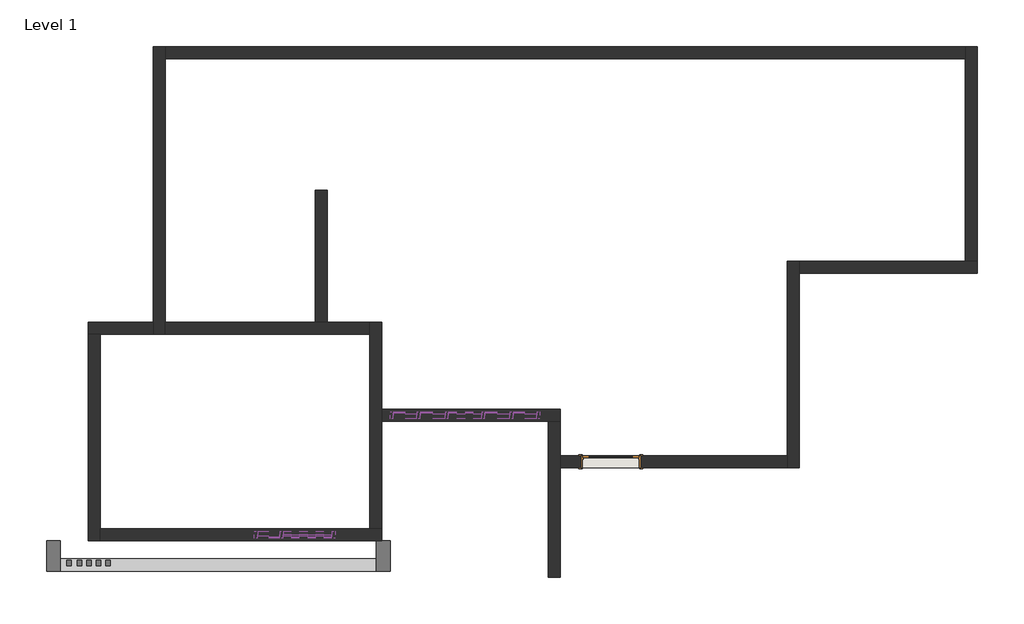
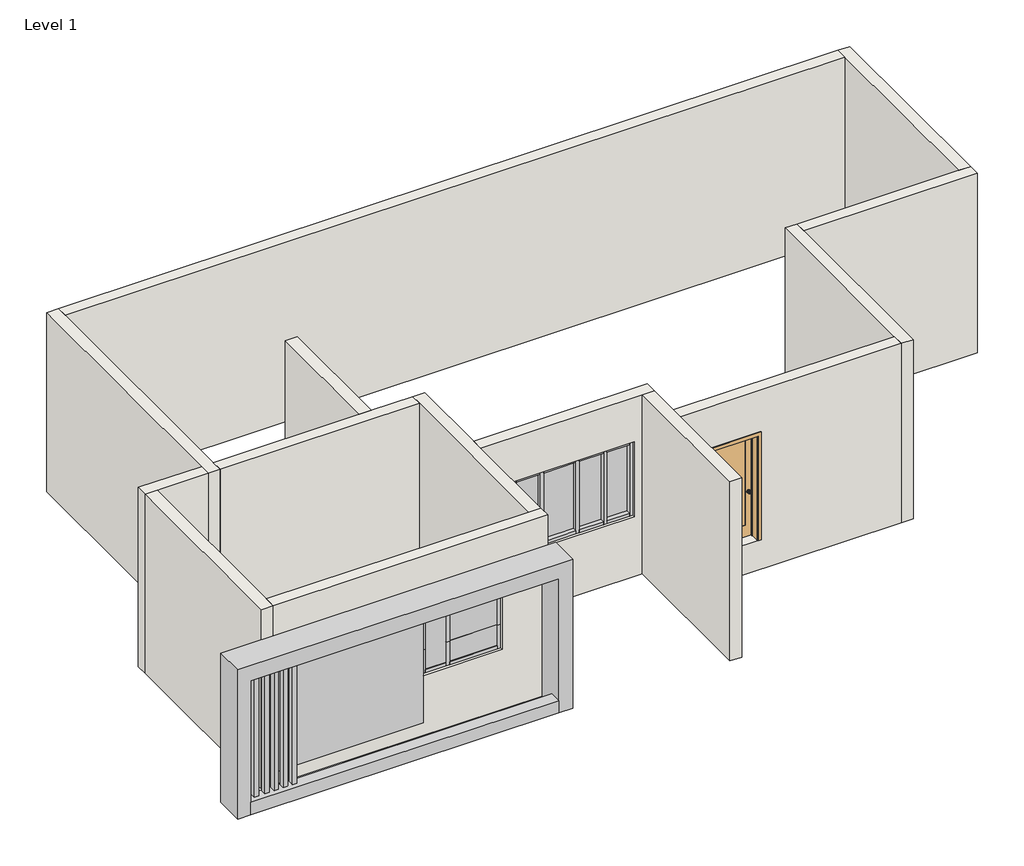
# One storey: 31 members, 14 walls, 9 plates, 1 door, 1 proxy.
"""IFC4 building model written with IfcOpenShell, lengths in millimetres."""

from ifc_helpers import new_model, si_unit, frame, origin, place, context, project, spatial, polyline, outline, extrude, faceted_brep, transform, mapped, element, save
from components import generic_models_1_generic_models_1_fa73b27a, door_0f538abb, member_df2e51ae, member_6fb4a552, member_82905deb, member_2b79973d, member_081e0693, member_4491d118, member_dc106669, member_ff82125d, member_323df77c, member_bc554fa6, member_86d06fe4, member_50cacee6, system_panel_glazed_04bc9dae, system_panel_glazed_113fdc6f, system_panel_glazed_5827f34b, system_panel_glazed_08f033f8, system_panel_glazed_aa4e1581, system_panel_glazed_b16bc715

model = new_model("IFC4")

# Units and contexts
model_context = context("Model", 3, world=origin())
ifc_project = project(units=[si_unit("LENGTHUNIT", "METRE", prefix="MILLI")], contexts=[model_context])

# Site, building, storey
site = spatial("IfcSite", under=ifc_project)
building = spatial("IfcBuilding", under=site)
storey = spatial("IfcBuildingStorey", under=building, Name="Level 1", Elevation=-609.6)

# Proxy
placement = place(None, origin())
generic_models_1_generic_models_1_shape = generic_models_1_generic_models_1_fa73b27a(model_context)
element("IfcBuildingElementProxy", 1, Name="Generic Models 1 : Generic Models 1", ObjectType="Generic Models 1 : Generic Models 1", at=placement, inside=storey, context=model_context, shape_type="MappedRepresentation", body=[
    mapped(generic_models_1_generic_models_1_shape, transform((0.0, 0.0, 0.0), x_axis=(1.0, 0.0, 0.0), y_axis=(0.0, 1.0, 0.0), z_axis=(0.0, 0.0, 1.0))),
])

# Door
door_shape = door_0f538abb(model_context)
element("IfcDoor", 2, ObjectType="Door-Interior-Single-1_Panel-Wood : 42\" x 84\"", at=placement, inside=storey, context=model_context, shape_type="MappedRepresentation", body=[
    mapped(door_shape, transform((-1951.8981007, 5916.5450124, 0.0), x_axis=(-1.0, 0.0, 0.0), y_axis=(0.0, -1.0, 0.0), z_axis=(0.0, 0.0, 1.0))),
])

# Members
member_shape = member_df2e51ae(model_context)
element("IfcMember", 3, ObjectType="Rectangular Mullion : 1\" Square", at=placement, inside=storey, context=model_context, shape_type="MappedRepresentation", body=[
    mapped(member_shape, transform((-8117.7481007, 4541.7700124, 1651.0), x_axis=(0.0, 0.0, 1.0), y_axis=(0.0, 1.0, 0.0), z_axis=(-1.0, 0.0, 0.0))),
])
element("IfcMember", 4, ObjectType="Rectangular Mullion : 1\" Square", at=placement, inside=storey, context=model_context, shape_type="MappedRepresentation", body=[
    mapped(member_shape, transform((-8117.7481007, 4541.7700124, 1092.2), x_axis=(0.0, 0.0, 1.0), y_axis=(0.0, 1.0, 0.0), z_axis=(-1.0, 0.0, 0.0))),
])
member_2_shape = member_6fb4a552(model_context)
element("IfcMember", 5, ObjectType="Rectangular Mullion : 2.5\" x 5\" rectangular", at=placement, inside=storey, context=model_context, shape_type="MappedRepresentation", body=[
    mapped(member_2_shape, transform((-3348.8981007, 6789.6700124, 2133.6), x_axis=(0.0, 0.0, 1.0), y_axis=(0.0, -1.0, 0.0), z_axis=(1.0, 0.0, 0.0))),
])
element("IfcMember", 6, ObjectType="Rectangular Mullion : 2.5\" x 5\" rectangular", at=placement, inside=storey, context=model_context, shape_type="MappedRepresentation", body=[
    mapped(member_2_shape, transform((-5603.1481007, 6789.6700124, 2133.6), x_axis=(0.0, 0.0, 1.0), y_axis=(0.0, -1.0, 0.0), z_axis=(1.0, 0.0, 0.0))),
])
element("IfcMember", 7, ObjectType="Rectangular Mullion : 2.5\" x 5\" rectangular", at=placement, inside=storey, context=model_context, shape_type="MappedRepresentation", body=[
    mapped(member_2_shape, transform((-6041.2981007, 6789.6700124, 609.6), x_axis=(0.0, 0.0, -1.0), y_axis=(0.0, -1.0, 0.0), z_axis=(-1.0, 0.0, 0.0))),
])
element("IfcMember", 8, ObjectType="Rectangular Mullion : 2.5\" x 5\" rectangular", at=placement, inside=storey, context=model_context, shape_type="MappedRepresentation", body=[
    mapped(member_2_shape, transform((-3787.0481007, 6789.6700124, 609.6), x_axis=(0.0, 0.0, -1.0), y_axis=(0.0, -1.0, 0.0), z_axis=(-1.0, 0.0, 0.0))),
])
member_3_shape = member_82905deb(model_context)
element("IfcMember", 9, ObjectType="Rectangular Mullion : 2.5\" x 5\" rectangular", at=placement, inside=storey, context=model_context, shape_type="MappedRepresentation", body=[
    mapped(member_3_shape, transform((-5571.3981007, 6789.6700124, 609.6), x_axis=(1.0, 0.0, 0.0), y_axis=(0.0, -1.0, 0.0), z_axis=(0.0, 0.0, -1.0))),
])
element("IfcMember", 10, ObjectType="Rectangular Mullion : 2.5\" x 5\" rectangular", at=placement, inside=storey, context=model_context, shape_type="MappedRepresentation", body=[
    mapped(member_3_shape, transform((-3818.7981007, 6789.6700124, 609.6), x_axis=(1.0, 0.0, 0.0), y_axis=(0.0, -1.0, 0.0), z_axis=(0.0, 0.0, -1.0))),
])
element("IfcMember", 11, ObjectType="Rectangular Mullion : 2.5\" x 5\" rectangular", at=placement, inside=storey, context=model_context, shape_type="MappedRepresentation", body=[
    mapped(member_3_shape, transform((-5037.9981007, 6789.6700124, 609.6), x_axis=(1.0, 0.0, 0.0), y_axis=(0.0, -1.0, 0.0), z_axis=(0.0, 0.0, -1.0))),
])
element("IfcMember", 12, ObjectType="Rectangular Mullion : 2.5\" x 5\" rectangular", at=placement, inside=storey, context=model_context, shape_type="MappedRepresentation", body=[
    mapped(member_3_shape, transform((-4352.1981007, 6789.6700124, 609.6), x_axis=(1.0, 0.0, 0.0), y_axis=(0.0, -1.0, 0.0), z_axis=(0.0, 0.0, -1.0))),
])
member_4_shape = member_2b79973d(model_context)
element("IfcMember", 13, ObjectType="Rectangular Mullion : 2.5\" x 5\" rectangular", at=placement, inside=storey, context=model_context, shape_type="MappedRepresentation", body=[
    mapped(member_4_shape, transform((-5539.6481007, 6789.6700124, 609.6), x_axis=(0.0, 0.0, -1.0), y_axis=(0.0, -1.0, 0.0), z_axis=(-1.0, 0.0, 0.0))),
])
element("IfcMember", 14, ObjectType="Rectangular Mullion : 2.5\" x 5\" rectangular", at=placement, inside=storey, context=model_context, shape_type="MappedRepresentation", body=[
    mapped(member_4_shape, transform((-4320.4481007, 6789.6700124, 609.6), x_axis=(0.0, 0.0, -1.0), y_axis=(0.0, -1.0, 0.0), z_axis=(-1.0, 0.0, 0.0))),
])
member_5_shape = member_081e0693(model_context)
element("IfcMember", 15, ObjectType="Rectangular Mullion : 2.5\" x 5\" rectangular", at=placement, inside=storey, context=model_context, shape_type="MappedRepresentation", body=[
    mapped(member_5_shape, transform((-5006.2481007, 6789.6700124, 609.6), x_axis=(0.0, 0.0, -1.0), y_axis=(0.0, -1.0, 0.0), z_axis=(-1.0, 0.0, 0.0))),
])
element("IfcMember", 16, ObjectType="Rectangular Mullion : 2.5\" x 5\" rectangular", at=placement, inside=storey, context=model_context, shape_type="MappedRepresentation", body=[
    mapped(member_4_shape, transform((-3850.5481007, 6789.6700124, 2133.6), x_axis=(0.0, 0.0, 1.0), y_axis=(0.0, -1.0, 0.0), z_axis=(1.0, 0.0, 0.0))),
])
element("IfcMember", 17, ObjectType="Rectangular Mullion : 2.5\" x 5\" rectangular", at=placement, inside=storey, context=model_context, shape_type="MappedRepresentation", body=[
    mapped(member_4_shape, transform((-5069.7481007, 6789.6700124, 2133.6), x_axis=(0.0, 0.0, 1.0), y_axis=(0.0, -1.0, 0.0), z_axis=(1.0, 0.0, 0.0))),
])
element("IfcMember", 18, ObjectType="Rectangular Mullion : 2.5\" x 5\" rectangular", at=placement, inside=storey, context=model_context, shape_type="MappedRepresentation", body=[
    mapped(member_5_shape, transform((-4383.9481007, 6789.6700124, 2133.6), x_axis=(0.0, 0.0, 1.0), y_axis=(0.0, -1.0, 0.0), z_axis=(1.0, 0.0, 0.0))),
])
member_6_shape = member_4491d118(model_context)
element("IfcMember", 19, ObjectType="Rectangular Mullion : 2.5\" x 5\" rectangular", at=placement, inside=storey, context=model_context, shape_type="MappedRepresentation", body=[
    mapped(member_6_shape, transform((-6104.7981007, 6789.6700124, 2133.6), x_axis=(-1.0, 0.0, 0.0), y_axis=(0.0, -1.0, 0.0), z_axis=(0.0, 0.0, 1.0))),
])
element("IfcMember", 20, ObjectType="Rectangular Mullion : 2.5\" x 5\" rectangular", at=placement, inside=storey, context=model_context, shape_type="MappedRepresentation", body=[
    mapped(member_6_shape, transform((-3285.3981007, 6789.6700124, 609.6), x_axis=(1.0, 0.0, 0.0), y_axis=(0.0, -1.0, 0.0), z_axis=(0.0, 0.0, -1.0))),
])
member_7_shape = member_dc106669(model_context)
element("IfcMember", 21, ObjectType="Rectangular Mullion : 2.5\" x 5\" rectangular", at=placement, inside=storey, context=model_context, shape_type="MappedRepresentation", body=[
    mapped(member_7_shape, transform((-8593.9981007, 4541.7700124, 2133.6), x_axis=(0.0, 0.0, 1.0), y_axis=(0.0, 1.0, 0.0), z_axis=(-1.0, 0.0, 0.0))),
])
member_8_shape = member_ff82125d(model_context)
element("IfcMember", 22, ObjectType="Rectangular Mullion : 2.5\" x 5\" rectangular", at=placement, inside=storey, context=model_context, shape_type="MappedRepresentation", body=[
    mapped(member_8_shape, transform((-7196.9981007, 4541.7700124, 609.6), x_axis=(0.0, 0.0, -1.0), y_axis=(0.0, 1.0, 0.0), z_axis=(1.0, 0.0, 0.0))),
])
member_9_shape = member_323df77c(model_context)
element("IfcMember", 23, ObjectType="Rectangular Mullion : 2.5\" x 5\" rectangular", at=placement, inside=storey, context=model_context, shape_type="MappedRepresentation", body=[
    mapped(member_9_shape, transform((-8149.4981007, 4541.7700124, 609.6), x_axis=(-1.0, 0.0, 0.0), y_axis=(0.0, 1.0, 0.0), z_axis=(0.0, 0.0, -1.0))),
])
element("IfcMember", 24, ObjectType="Rectangular Mullion : 2.5\" x 5\" rectangular", at=placement, inside=storey, context=model_context, shape_type="MappedRepresentation", body=[
    mapped(member_7_shape, transform((-8181.2481007, 4541.7700124, 609.6), x_axis=(0.0, 0.0, -1.0), y_axis=(0.0, 1.0, 0.0), z_axis=(1.0, 0.0, 0.0))),
])
element("IfcMember", 25, ObjectType="Rectangular Mullion : 2.5\" x 5\" rectangular", at=placement, inside=storey, context=model_context, shape_type="MappedRepresentation", body=[
    mapped(member_8_shape, transform((-8117.7481007, 4541.7700124, 2133.6), x_axis=(0.0, 0.0, 1.0), y_axis=(0.0, 1.0, 0.0), z_axis=(-1.0, 0.0, 0.0))),
])
member_10_shape = member_bc554fa6(model_context)
element("IfcMember", 26, ObjectType="Rectangular Mullion : 2.5\" x 5\" rectangular", at=placement, inside=storey, context=model_context, shape_type="MappedRepresentation", body=[
    mapped(member_10_shape, transform((-8149.4981007, 4541.7700124, 1092.2), x_axis=(-1.0, 0.0, 0.0), y_axis=(0.0, 1.0, 0.0), z_axis=(0.0, 0.0, -1.0))),
])
element("IfcMember", 27, ObjectType="Rectangular Mullion : 2.5\" x 5\" rectangular", at=placement, inside=storey, context=model_context, shape_type="MappedRepresentation", body=[
    mapped(member_9_shape, transform((-8149.4981007, 4541.7700124, 1651.0), x_axis=(-1.0, 0.0, 0.0), y_axis=(0.0, 1.0, 0.0), z_axis=(0.0, 0.0, -1.0))),
])
member_11_shape = member_86d06fe4(model_context)
element("IfcMember", 28, ObjectType="Rectangular Mullion : 2.5\" x 5\" rectangular", at=placement, inside=storey, context=model_context, shape_type="MappedRepresentation", body=[
    mapped(member_11_shape, transform((-7133.4981007, 4541.7700124, 2133.6), x_axis=(1.0, 0.0, 0.0), y_axis=(0.0, 1.0, 0.0), z_axis=(0.0, 0.0, 1.0))),
])
element("IfcMember", 29, ObjectType="Rectangular Mullion : 2.5\" x 5\" rectangular", at=placement, inside=storey, context=model_context, shape_type="MappedRepresentation", body=[
    mapped(member_11_shape, transform((-8657.4981007, 4541.7700124, 609.6), x_axis=(-1.0, 0.0, 0.0), y_axis=(0.0, 1.0, 0.0), z_axis=(0.0, 0.0, -1.0))),
])
member_12_shape = member_50cacee6(model_context)
element("IfcMember", 30, ObjectType="Rectangular Mullion : 2.5\" x 5\" rectangular", at=placement, inside=storey, context=model_context, shape_type="MappedRepresentation", body=[
    mapped(member_12_shape, transform((-8657.4981007, 4541.7700124, 1092.2), x_axis=(-1.0, 0.0, 0.0), y_axis=(0.0, 1.0, 0.0), z_axis=(0.0, 0.0, -1.0))),
])
element("IfcMember", 31, ObjectType="Rectangular Mullion : 2.5\" x 5\" rectangular", at=placement, inside=storey, context=model_context, shape_type="MappedRepresentation", body=[
    mapped(member_11_shape, transform((-8657.4981007, 4541.7700124, 1651.0), x_axis=(-1.0, 0.0, 0.0), y_axis=(0.0, 1.0, 0.0), z_axis=(0.0, 0.0, -1.0))),
])
element("IfcMember", 32, ObjectType="Rectangular Mullion : 2.5\" x 5\" rectangular", at=placement, inside=storey, context=model_context, shape_type="MappedRepresentation", body=[
    mapped(member_11_shape, transform((-7133.4981007, 4541.7700124, 1092.2), x_axis=(1.0, 0.0, 0.0), y_axis=(0.0, 1.0, 0.0), z_axis=(0.0, 0.0, 1.0))),
])
element("IfcMember", 33, ObjectType="Rectangular Mullion : 2.5\" x 5\" rectangular", at=placement, inside=storey, context=model_context, shape_type="MappedRepresentation", body=[
    mapped(member_12_shape, transform((-7133.4981007, 4541.7700124, 1651.0), x_axis=(1.0, 0.0, 0.0), y_axis=(0.0, 1.0, 0.0), z_axis=(0.0, 0.0, 1.0))),
])

# Plates
system_panel_glazed_shape = system_panel_glazed_04bc9dae(model_context)
element("IfcPlate", 34, ObjectType="System Panel : Glazed", at=placement, inside=storey, context=model_context, shape_type="MappedRepresentation", body=[
    mapped(system_panel_glazed_shape, transform((-5822.2231007, 6789.6700124, 673.1), x_axis=(1.0, 0.0, 0.0), y_axis=(0.0, 1.0, 0.0), z_axis=(0.0, 0.0, 1.0))),
])
element("IfcPlate", 35, ObjectType="System Panel : Glazed", at=placement, inside=storey, context=model_context, shape_type="MappedRepresentation", body=[
    mapped(system_panel_glazed_shape, transform((-3567.9731007, 6789.6700124, 673.1), x_axis=(1.0, 0.0, 0.0), y_axis=(0.0, 1.0, 0.0), z_axis=(0.0, 0.0, 1.0))),
])
system_panel_glazed_2_shape = system_panel_glazed_113fdc6f(model_context)
element("IfcPlate", 36, ObjectType="System Panel : Glazed", at=placement, inside=storey, context=model_context, shape_type="MappedRepresentation", body=[
    mapped(system_panel_glazed_2_shape, transform((-5304.6981007, 6789.6700124, 673.1), x_axis=(1.0, 0.0, 0.0), y_axis=(0.0, 1.0, 0.0), z_axis=(0.0, 0.0, 1.0))),
])
element("IfcPlate", 37, ObjectType="System Panel : Glazed", at=placement, inside=storey, context=model_context, shape_type="MappedRepresentation", body=[
    mapped(system_panel_glazed_2_shape, transform((-4085.4981007, 6789.6700124, 673.1), x_axis=(1.0, 0.0, 0.0), y_axis=(0.0, 1.0, 0.0), z_axis=(0.0, 0.0, 1.0))),
])
system_panel_glazed_3_shape = system_panel_glazed_5827f34b(model_context)
element("IfcPlate", 38, ObjectType="System Panel : Glazed", at=placement, inside=storey, context=model_context, shape_type="MappedRepresentation", body=[
    mapped(system_panel_glazed_3_shape, transform((-4695.0981007, 6789.6700124, 673.1), x_axis=(1.0, 0.0, 0.0), y_axis=(0.0, 1.0, 0.0), z_axis=(0.0, 0.0, 1.0))),
])
system_panel_glazed_4_shape = system_panel_glazed_08f033f8(model_context)
element("IfcPlate", 39, ObjectType="System Panel : Glazed", at=placement, inside=storey, context=model_context, shape_type="MappedRepresentation", body=[
    mapped(system_panel_glazed_4_shape, transform((-7657.3731007, 4541.7700124, 673.1), x_axis=(-1.0, 0.0, 0.0), y_axis=(0.0, -1.0, 0.0), z_axis=(0.0, 0.0, 1.0))),
])
element("IfcPlate", 40, ObjectType="System Panel : Glazed", at=placement, inside=storey, context=model_context, shape_type="MappedRepresentation", body=[
    mapped(system_panel_glazed_4_shape, transform((-7657.3731007, 4541.7700124, 1651.0), x_axis=(-1.0, 0.0, 0.0), y_axis=(0.0, -1.0, 0.0), z_axis=(0.0, 0.0, 1.0))),
])
system_panel_glazed_5_shape = system_panel_glazed_aa4e1581(model_context)
element("IfcPlate", 41, ObjectType="System Panel : Glazed", at=placement, inside=storey, context=model_context, shape_type="MappedRepresentation", body=[
    mapped(system_panel_glazed_5_shape, transform((-8387.6231007, 4541.7700124, 673.1), x_axis=(-1.0, 0.0, 0.0), y_axis=(0.0, -1.0, 0.0), z_axis=(0.0, 0.0, 1.0))),
])
system_panel_glazed_6_shape = system_panel_glazed_b16bc715(model_context)
element("IfcPlate", 42, ObjectType="System Panel : Glazed", at=placement, inside=storey, context=model_context, shape_type="MappedRepresentation", body=[
    mapped(system_panel_glazed_6_shape, transform((-7657.3731007, 4541.7700124, 1092.2), x_axis=(-1.0, 0.0, 0.0), y_axis=(0.0, -1.0, 0.0), z_axis=(0.0, 0.0, 1.0))),
])

# Walls
element("IfcWall", 43, ObjectType="9\" wall", at=placement, inside=storey, context=model_context, shape_type="Brep", body=[
    faceted_brep([(-10562.4981007, 13723.8700124, -609.6), (-10562.4981007, 8542.2700124, -609.6), (-10562.4981007, 8313.6700124, -609.6), (-10562.4981007, 8313.6700124, 3048.0), (-10562.4981007, 8542.2700124, 3048.0), (-10562.4981007, 13723.8700124, 3048.0), (-10333.8981007, 13723.8700124, -609.6), (-10333.8981007, 13723.8700124, 3048.0), (-10333.8981007, 13495.2700124, 3048.0), (-10333.8981007, 8542.2700124, 3048.0), (-10333.8981007, 8313.6700124, 3048.0), (-10333.8981007, 8313.6700124, -609.6), (-10333.8981007, 8542.2700124, -609.6), (-10333.8981007, 13495.2700124, -609.6)], [[[0, 1, 2, 3, 4, 5]], [[6, 7, 8, 9, 10, 11, 12, 13]], [[2, 1, 0, 6, 13, 12, 11]], [[5, 4, 3, 10, 9, 8, 7]], [[3, 2, 11, 10]], [[0, 5, 7, 6]]]),
])
element("IfcWall", 44, ObjectType="9\" wall", at=placement, inside=storey, context=model_context, shape_type="Brep", body=[
    faceted_brep([(-10562.4981007, 8542.2700124, -609.6), (-11781.6981007, 8542.2700124, -609.6), (-11781.6981007, 8542.2700124, 3048.0), (-10562.4981007, 8542.2700124, 3048.0), (-10562.4981007, 8313.6700124, -609.6), (-10562.4981007, 8313.6700124, 3048.0), (-11553.0981007, 8313.6700124, 3048.0), (-11781.6981007, 8313.6700124, 3048.0), (-11781.6981007, 8313.6700124, -609.6), (-11553.0981007, 8313.6700124, -609.6)], [[[0, 1, 2, 3]], [[4, 5, 6, 7, 8, 9]], [[1, 0, 4, 9, 8]], [[3, 2, 7, 6, 5]], [[0, 3, 5, 4]], [[2, 1, 8, 7]]]),
])
element("IfcWall", 45, ObjectType="9\" wall", at=placement, inside=storey, context=model_context, shape_type="Brep", body=[
    faceted_brep([(-11781.6981007, 8313.6700124, -609.6), (-11781.6981007, 4427.4700124, -609.6), (-11781.6981007, 4427.4700124, 3048.0), (-11781.6981007, 8313.6700124, 3048.0), (-11553.0981007, 8313.6700124, -609.6), (-11553.0981007, 8313.6700124, 3048.0), (-11553.0981007, 4656.0700124, 3048.0), (-11553.0981007, 4427.4700124, 3048.0), (-11553.0981007, 4427.4700124, -609.6), (-11553.0981007, 4656.0700124, -609.6)], [[[0, 1, 2, 3]], [[4, 5, 6, 7, 8, 9]], [[1, 0, 4, 9, 8]], [[3, 2, 7, 6, 5]], [[0, 3, 5, 4]], [[2, 1, 8, 7]]]),
])
element("IfcWall", 46, ObjectType="9\" wall", at=placement, inside=storey, context=model_context, shape_type="Brep", body=[
    faceted_brep([(-11553.0981007, 4427.4700124, -609.6), (-6257.1981007, 4427.4700124, -609.6), (-6257.1981007, 4427.4700124, 3048.0), (-11553.0981007, 4427.4700124, 3048.0), (-7133.4981007, 4427.4700124, 2133.6), (-7133.4981007, 4427.4700124, 609.6), (-8657.4981007, 4427.4700124, 609.6), (-8657.4981007, 4427.4700124, 2133.6), (-6257.1981007, 4656.0700124, -609.6), (-6485.7981007, 4656.0700124, -609.6), (-11553.0981007, 4656.0700124, -609.6), (-11553.0981007, 4656.0700124, 3048.0), (-6485.7981007, 4656.0700124, 3048.0), (-6257.1981007, 4656.0700124, 3048.0), (-7133.4981007, 4656.0700124, 609.6), (-7133.4981007, 4656.0700124, 2133.6), (-8657.4981007, 4656.0700124, 2133.6), (-8657.4981007, 4656.0700124, 609.6)], [[[0, 1, 2, 3], [4, 5, 6, 7]], [[8, 9, 10, 11, 12, 13], [14, 15, 16, 17]], [[1, 0, 10, 9, 8]], [[3, 2, 13, 12, 11]], [[0, 3, 11, 10]], [[2, 1, 8, 13]], [[14, 5, 4, 15]], [[15, 4, 7, 16]], [[16, 7, 6, 17]], [[5, 14, 17, 6]]]),
])
element("IfcWall", 47, ObjectType="9\" wall", at=placement, inside=storey, context=model_context, shape_type="Brep", body=[
    faceted_brep([(-6257.1981007, 4656.0700124, -609.6), (-6257.1981007, 6675.3700124, -609.6), (-6257.1981007, 6903.9700124, -609.6), (-6257.1981007, 8542.2700124, -609.6), (-6257.1981007, 8542.2700124, 3048.0), (-6257.1981007, 6903.9700124, 3048.0), (-6257.1981007, 6675.3700124, 3048.0), (-6257.1981007, 4656.0700124, 3048.0), (-6485.7981007, 4656.0700124, -609.6), (-6485.7981007, 4656.0700124, 3048.0), (-6485.7981007, 8313.6700124, 3048.0), (-6485.7981007, 8542.2700124, 3048.0), (-6485.7981007, 8542.2700124, -609.6), (-6485.7981007, 8313.6700124, -609.6)], [[[0, 1, 2, 3, 4, 5, 6, 7]], [[8, 9, 10, 11, 12, 13]], [[3, 2, 1, 0, 8, 13, 12]], [[7, 6, 5, 4, 11, 10, 9]], [[0, 7, 9, 8]], [[4, 3, 12, 11]]]),
])
element("IfcWall", 48, ObjectType="9\" wall", at=placement, inside=storey, context=model_context, shape_type="Brep", body=[
    faceted_brep([(-10333.8981007, 8313.6700124, -609.6), (-6485.7981007, 8313.6700124, -609.6), (-6485.7981007, 8313.6700124, 3048.0), (-10333.8981007, 8313.6700124, 3048.0), (-10333.8981007, 8542.2700124, -609.6), (-10333.8981007, 8542.2700124, 3048.0), (-7514.4981007, 8542.2700124, 3048.0), (-7285.8981007, 8542.2700124, 3048.0), (-6485.7981007, 8542.2700124, 3048.0), (-6485.7981007, 8542.2700124, -609.6), (-7285.8981007, 8542.2700124, -609.6), (-7514.4981007, 8542.2700124, -609.6)], [[[0, 1, 2, 3]], [[4, 5, 6, 7, 8, 9, 10, 11]], [[1, 0, 4, 11, 10, 9]], [[3, 2, 8, 7, 6, 5]], [[0, 3, 5, 4]], [[2, 1, 9, 8]]]),
])
element("IfcWall", 49, ObjectType="9\" wall", at=placement, inside=storey, context=model_context, shape_type="SweptSolid", body=[
    extrude(outline(polyline([(-7285.8981007, 11018.7700124), (-7285.8981007, 8542.2700124), (-7514.4981007, 8542.2700124), (-7514.4981007, 11018.7700124), (-7285.8981007, 11018.7700124)])), frame((0.0, 0.0, -609.6), z_axis=(0.0, 0.0, 1.0), x_axis=(1.0, 0.0, 0.0)), (0.0, 0.0, 1.0), 3657.6),
])
element("IfcWall", 50, ObjectType="9\" wall", at=placement, inside=storey, context=model_context, shape_type="Brep", body=[
    faceted_brep([(-6257.1981007, 6675.3700124, -609.6), (-3132.9981007, 6675.3700124, -609.6), (-2904.3981007, 6675.3700124, -609.6), (-2904.3981007, 6675.3700124, 3048.0), (-3132.9981007, 6675.3700124, 3048.0), (-6257.1981007, 6675.3700124, 3048.0), (-6104.7981007, 6675.3700124, 609.6), (-6104.7981007, 6675.3700124, 2133.6), (-3285.3981007, 6675.3700124, 2133.6), (-3285.3981007, 6675.3700124, 609.6), (-2904.3981007, 6903.9700124, -609.6), (-6257.1981007, 6903.9700124, -609.6), (-6257.1981007, 6903.9700124, 3048.0), (-2904.3981007, 6903.9700124, 3048.0), (-6104.7981007, 6903.9700124, 2133.6), (-6104.7981007, 6903.9700124, 609.6), (-3285.3981007, 6903.9700124, 609.6), (-3285.3981007, 6903.9700124, 2133.6)], [[[0, 1, 2, 3, 4, 5], [6, 7, 8, 9]], [[10, 11, 12, 13], [14, 15, 16, 17]], [[2, 1, 0, 11, 10]], [[5, 4, 3, 13, 12]], [[0, 5, 12, 11]], [[3, 2, 10, 13]], [[6, 15, 14, 7]], [[7, 14, 17, 8]], [[8, 17, 16, 9]], [[15, 6, 9, 16]]]),
])
element("IfcWall", 51, ObjectType="9\" wall", at=placement, inside=storey, context=model_context, shape_type="Brep", body=[
    faceted_brep([(-3132.9981007, 6675.3700124, -609.6), (-3132.9981007, 3741.6700124, -609.6), (-3132.9981007, 3741.6700124, 3048.0), (-3132.9981007, 6675.3700124, 3048.0), (-2904.3981007, 6675.3700124, -609.6), (-2904.3981007, 6675.3700124, 3048.0), (-2904.3981007, 6027.6700124, 3048.0), (-2904.3981007, 5799.0700124, 3048.0), (-2904.3981007, 3741.6700124, 3048.0), (-2904.3981007, 3741.6700124, -609.6), (-2904.3981007, 5799.0700124, -609.6), (-2904.3981007, 6027.6700124, -609.6)], [[[0, 1, 2, 3]], [[4, 5, 6, 7, 8, 9, 10, 11]], [[1, 0, 4, 11, 10, 9]], [[2, 1, 9, 8]], [[3, 2, 8, 7, 6, 5]], [[0, 3, 5, 4]]]),
])
element("IfcWall", 52, ObjectType="9\" wall", at=placement, inside=storey, context=model_context, shape_type="Brep", body=[
    faceted_brep([(1591.4018993, 5799.0700124, -609.6), (1591.4018993, 9456.6700124, -609.6), (1591.4018993, 9685.2700124, -609.6), (1591.4018993, 9685.2700124, 3048.0), (1591.4018993, 9456.6700124, 3048.0), (1591.4018993, 5799.0700124, 3048.0), (1362.8018993, 5799.0700124, -609.6), (1362.8018993, 5799.0700124, 3048.0), (1362.8018993, 6027.6700124, 3048.0), (1362.8018993, 9685.2700124, 3048.0), (1362.8018993, 9685.2700124, -609.6), (1362.8018993, 6027.6700124, -609.6)], [[[0, 1, 2, 3, 4, 5]], [[6, 7, 8, 9, 10, 11]], [[2, 1, 0, 6, 11, 10]], [[5, 4, 3, 9, 8, 7]], [[3, 2, 10, 9]], [[0, 5, 7, 6]]]),
])
element("IfcWall", 53, ObjectType="9\" wall", at=placement, inside=storey, context=model_context, shape_type="Brep", body=[
    faceted_brep([(1591.4018993, 9456.6700124, -609.6), (4944.2018993, 9456.6700124, -609.6), (4944.2018993, 9456.6700124, 3048.0), (1591.4018993, 9456.6700124, 3048.0), (1591.4018993, 9685.2700124, -609.6), (1591.4018993, 9685.2700124, 3048.0), (4715.6018993, 9685.2700124, 3048.0), (4944.2018993, 9685.2700124, 3048.0), (4944.2018993, 9685.2700124, -609.6), (4715.6018993, 9685.2700124, -609.6)], [[[0, 1, 2, 3]], [[4, 5, 6, 7, 8, 9]], [[1, 0, 4, 9, 8]], [[3, 2, 7, 6, 5]], [[0, 3, 5, 4]], [[2, 1, 8, 7]]]),
])
element("IfcWall", 54, ObjectType="9\" wall", at=placement, inside=storey, context=model_context, shape_type="Brep", body=[
    faceted_brep([(4944.2018993, 9685.2700124, -609.6), (4944.2018993, 13723.8700124, -609.6), (4944.2018993, 13723.8700124, 3048.0), (4944.2018993, 9685.2700124, 3048.0), (4715.6018993, 9685.2700124, -609.6), (4715.6018993, 9685.2700124, 3048.0), (4715.6018993, 13495.2700124, 3048.0), (4715.6018993, 13723.8700124, 3048.0), (4715.6018993, 13723.8700124, -609.6), (4715.6018993, 13495.2700124, -609.6)], [[[0, 1, 2, 3]], [[4, 5, 6, 7, 8, 9]], [[1, 0, 4, 9, 8]], [[3, 2, 7, 6, 5]], [[0, 3, 5, 4]], [[2, 1, 8, 7]]]),
])
element("IfcWall", 55, ObjectType="9\" wall", at=placement, inside=storey, context=model_context, shape_type="SweptSolid", body=[
    extrude(outline(polyline([(-10333.8981007, 13723.8700124), (4715.6018993, 13723.8700124), (4715.6018993, 13495.2700124), (-10333.8981007, 13495.2700124), (-10333.8981007, 13723.8700124)])), frame((0.0, 0.0, -609.6), z_axis=(0.0, 0.0, 1.0), x_axis=(1.0, 0.0, 0.0)), (0.0, 0.0, 1.0), 3657.6),
])
element("IfcWall", 56, ObjectType="9\" wall", at=placement, inside=storey, context=model_context, shape_type="SweptSolid", body=[
    extrude(outline(polyline([(-609.6, -2904.3981007), (-609.6, 1362.8018993), (3048.0, 1362.8018993), (3048.0, -2904.3981007), (-609.6, -2904.3981007)]), holes=[polyline([(0.0, -2510.6981007), (2159.0, -2510.6981007), (2159.0, -1393.0981007), (0.0, -1393.0981007), (0.0, -2510.6981007)])]), frame((0.0, 5799.0700124, 0.0), z_axis=(0.0, 1.0, 0.0), x_axis=(0.0, 0.0, 1.0)), (0.0, 0.0, 1.0), 228.6),
])

save(model, "model.ifc")

# Revit data of these elements
# Type "Door-Interior-Single-1_Panel-Wood : 42\" x 84\""
#   Type Mark = "9"
#   Assembly Code = "C1020300"
#   Analytic Construction = "Wooden"
#   Top Rail = 0' - 4 11/16"
#   Thickness = 0' - 1 3/8"
#   Thermal Resistance (R) = 2.5876 (h·ft²·°F)/BTU
#   Swing Angle [instance default] = 90.00°
#   Stiles = 0' - 4 3/4"
#   Rough Width = 3' - 8"
#   Rough Height = 7' - 1"
#   Height = 7' - 0"
#   Width = 3' - 6"
#   Heat Transfer Coefficient (U) = 0.3865 BTU/(h·ft²·°F)
#   Bottom Rail = 0' - 9 1/8"
#   Trim Material = Cherry
#   Panel Material = Cherry
#   Frame Material = Cherry
#   Door Handle Material = Aluminum
#   Visual Light Transmittance = 0
#   Solar Heat Gain Coefficient = 0
#   Wall Closure = (empty or 0)
#   Function = (empty or 0)
# Type "Rectangular Mullion : 1\" Square"
#   built-in parameter 1007304 = 0.0833333 (stored number, unit not read)
#   built-in parameter 1007301 = 0.0416667 (stored number, unit not read)
#   built-in parameter 1007300 = 0.0416667 (stored number, unit not read)
# Type "Rectangular Mullion : 2.5\" x 5\" rectangular"
#   built-in parameter 1007304 = 0.416667 (stored number, unit not read)
#   built-in parameter 1007301 = 0.104167 (stored number, unit not read)
#   built-in parameter 1007300 = 0.104167 (stored number, unit not read)
# Type "System Panel : Glazed"
#   Construction Type Id = "GSP4R"
#   Analytic Construction = "1/8 in Pilkington single glazing"
#   Visual Light Transmittance = 0.9
#   Solar Heat Gain Coefficient = 0.86
#   Heat Transfer Coefficient (U) = 1.18115 BTU/(h·ft²·°F)
#   Define Thermal Properties by = 1
# Type "9\" wall"
#   Assembly Code = "B2010"
#   Layers, outside or top first: 0' - 9" no material (function 1)
# Element 1 (IfcBuildingElementProxy, "Generic Models 1 : Generic Models 1")
#   Phase Created = New Construction
# Element 2 (IfcDoor, "Door-Interior-Single-1_Panel-Wood : 42\" x 84\"")
#   Swing Angle = 90.00°
#   Phase Created = New Construction
#   Materials on its faces: "Cherry", "Aluminum"
# Elements 3, 4 (IfcMember, "Rectangular Mullion : 1\" Square")
#   Phase Created = New Construction
#   Materials on its faces: "Rectangle 1 sq"
# Elements 5, 6, 7, 8, 9, 10, 11, 12, 13, 14, 15, 16, 17, 18, 19, 20, 21, 22, 23, 24, 25, 26, 27, 28, 29, 30, 31, 32, 33 (IfcMember, "Rectangular Mullion : 2.5\" x 5\" rectangular")
#   Phase Created = New Construction
#   Materials on its faces: "Rectangle 1 sq"
# Elements 34, 35, 36, 37, 38, 39, 40, 41, 42 (IfcPlate, "System Panel : Glazed")
#   Phase Created = New Construction
#   Materials on its faces: "Glass"
# Elements 43, 44, 45, 46, 47, 48, 49, 50, 51, 52, 53, 54, 55, 56 (IfcWall, "9\" wall")
#   Top Offset = 0' - 0"
#   Base Offset = 0' - 0"
#   wall height = 12' - 0"
#   Phase Created = New Construction
#   Base Constraint = Level 1
#   Top Constraint = Level 2
#   Materials on its faces: "Default Wall"
# Materials
#   "Cherry": class "Wood", colour RGB 226 177 128, transparency 0, Description = "Prunus Serotina", Cost = 0
#   "Aluminum": class "Metal", colour RGB 247 247 247, transparency 0, Description = "Aluminum 6061", Cost = 0
#   "Rectangle 1 sq": class "Generic", colour RGB 120 120 120, transparency 0, Cost = 0
#   "Glass": class "Glass", colour RGB 0 128 192, transparency 0.75, Description = "Soda Lime Glass", Cost = 0
#   "Default Wall": colour RGB 128 128 128, transparency 0, Cost = 0
